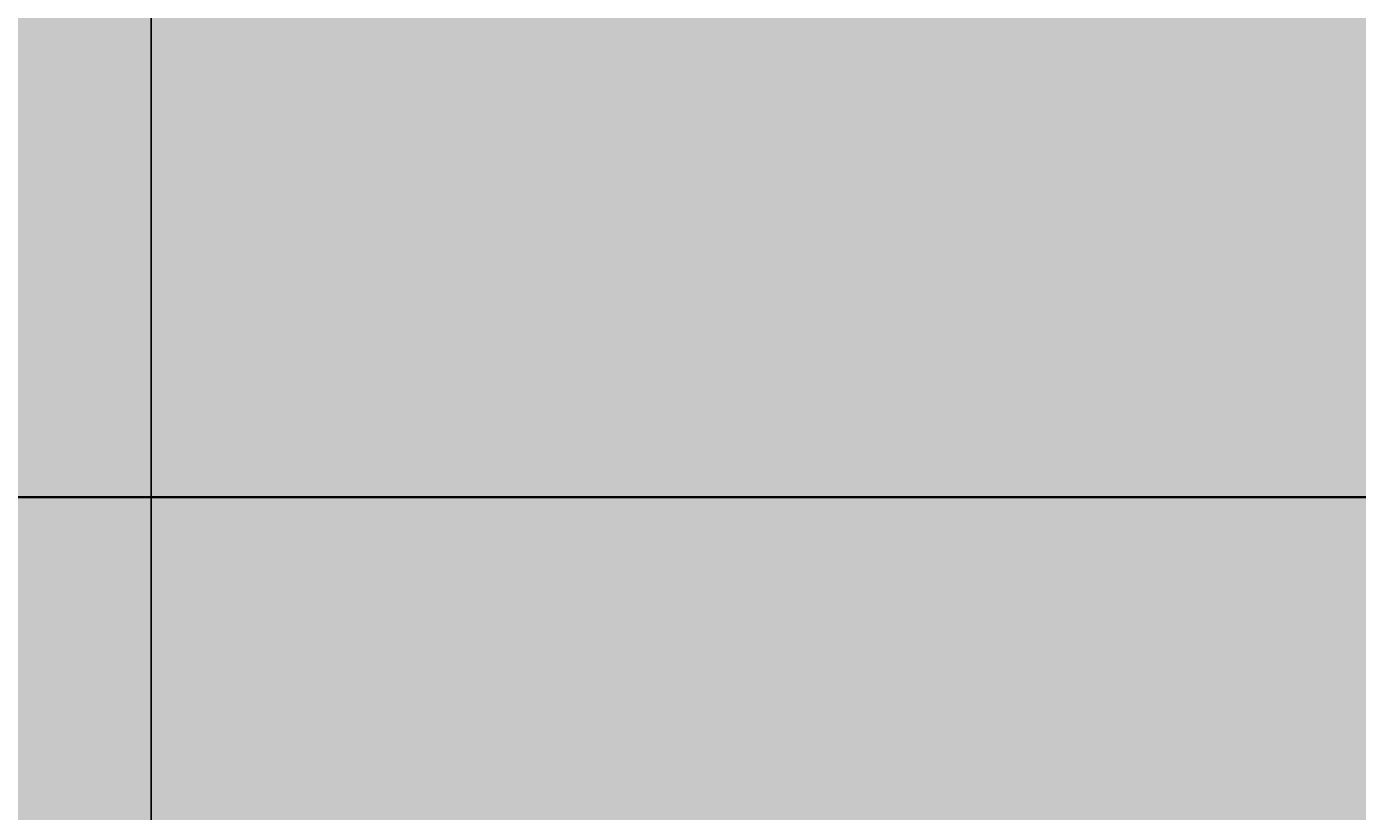
# Model space of a CAD drawing. Units: feet. Extents: x 2695 to 2912, y 795 to 1139.
# Tile 76 of 83: x 2840 to 2876, y 1042 to 1063. Entities that reach past the tile are written whole.
import ezdxf

# ---------------------------------------------------------------- set-up
doc = ezdxf.new("R2010")
doc.units = ezdxf.units.FT
for name, color, linetype, lineweight in [('A-ANNO-DIMS', 2, 'Continuous', 18), ('A-ELEV', 7, 'Continuous', 35), ('A-ELEV-PATT', 252, 'Continuous', 13)]:
    doc.layers.add(name, color=color, linetype=linetype, lineweight=lineweight)
doc.styles.get("Standard").update_dxf_attribs({"font": 'arial.ttf'})
doc.dimstyles.get("Standard").update_dxf_attribs({"dimtxt": 0.18, "dimasz": 0.18, "dimexe": 0.18, "dimexo": 0.0625, "dimgap": 0.09, "dimtad": 0, "dimtih": 1, "dimtoh": 1, "dimdec": 1, "dimzin": 0, "dimdsep": 46, "dimlunit": 3, "dimtxsty": 'Standard', "dimcen": 0.09, "dimadec": 0, "dimazin": 0, "dimtfac": 1, "dimtdec": 1, "dimtofl": 0, "dimtmove": 0, "dimatfit": 3, "dimfxl": 1, "dimtolj": 1, "dimtzin": 0, "dimarcsym": 0})

# ---------------------------------------------------------------- blocks, each defined once
blk = doc.blocks.new('*D10')
at = {"layer": 'A-ANNO-DIMS', "color": 0, "lineweight": -2, "transparency": 16777216}
for p, q in [((2778.034, 1020.886), (2778.034, 1138.886)), ((2778.214, 1138.706), (2810.411, 1138.706)), ((2843.395, 1138.706), (2811.198, 1138.706)), ((2843.575, 1020.886), (2843.575, 1138.886))]:
    blk.add_line(p, q, dxfattribs=at)
at = {"layer": 'A-ANNO-DIMS', "color": 0, "transparency": 16777216}
for points in [[(2778.214, 1138.736), (2778.214, 1138.676), (2778.034, 1138.706)], [(2843.395, 1138.736), (2843.395, 1138.676), (2843.575, 1138.706)]]:
    blk.add_solid(points, dxfattribs=at)
at = {"layer": 'Defpoints', "color": 0, "transparency": 16777216}
for p in [(2843.575, 1138.706), (2778.034, 1020.824), (2843.575, 1020.824)]:
    blk.add_point(p, dxfattribs=at)
at = {"layer": 'A-ANNO-DIMS', "color": 0, "transparency": 16777216, "insert": (2810.805, 1138.706), "char_height": 0.18, "attachment_point": 5}
blk.add_mtext('\\A1;65.54', dxfattribs=at)
blk = doc.blocks.new('*D11')
at = {"layer": 'A-ANNO-DIMS', "color": 0, "lineweight": -2, "transparency": 16777216}
for p, q in [((2843.575, 1020.886), (2843.575, 1138.886)), ((2843.755, 1138.706), (2869.128, 1138.706)), ((2895.289, 1138.706), (2869.916, 1138.706)), ((2895.469, 1107.898), (2895.469, 1138.886))]:
    blk.add_line(p, q, dxfattribs=at)
at = {"layer": 'A-ANNO-DIMS', "color": 0, "transparency": 16777216}
for points in [[(2843.755, 1138.736), (2843.755, 1138.676), (2843.575, 1138.706)], [(2895.289, 1138.736), (2895.289, 1138.676), (2895.469, 1138.706)]]:
    blk.add_solid(points, dxfattribs=at)
at = {"layer": 'Defpoints', "color": 0, "transparency": 16777216}
for p in [(2895.469, 1138.706), (2895.469, 1107.835), (2843.575, 1020.824)]:
    blk.add_point(p, dxfattribs=at)
at = {"layer": 'A-ANNO-DIMS', "color": 0, "transparency": 16777216, "insert": (2869.522, 1138.706), "char_height": 0.18, "attachment_point": 5}
blk.add_mtext('\\A1;51.89', dxfattribs=at)
blk = doc.blocks.new('*D18')
at = {"layer": 'A-ANNO-DIMS', "color": 0, "lineweight": -2, "transparency": 16777216}
for p, q in [((2890.699, 1050.311), (2911.424, 1050.311)), ((2911.244, 1050.131), (2911.244, 1035.749)), ((2911.244, 1021.004), (2911.244, 1035.385)), ((2843.637, 1020.824), (2911.424, 1020.824))]:
    blk.add_line(p, q, dxfattribs=at)
at = {"layer": 'A-ANNO-DIMS', "color": 0, "transparency": 16777216}
for points in [[(2911.214, 1050.131), (2911.274, 1050.131), (2911.244, 1050.311)], [(2911.214, 1021.004), (2911.274, 1021.004), (2911.244, 1020.824)]]:
    blk.add_solid(points, dxfattribs=at)
at = {"layer": 'Defpoints', "color": 0, "transparency": 16777216}
for p in [(2890.636, 1050.311), (2911.244, 1050.311), (2843.575, 1020.824)]:
    blk.add_point(p, dxfattribs=at)
at = {"layer": 'A-ANNO-DIMS', "color": 0, "transparency": 16777216, "insert": (2911.244, 1035.567), "char_height": 0.18, "attachment_point": 5}
blk.add_mtext('\\A1;29.487', dxfattribs=at)
blk = doc.blocks.new('*D50')
at = {"layer": 'A-ANNO-DIMS', "color": 0, "lineweight": -2, "transparency": 16777216}
for p, q in [((2810.041, 972.03), (2810.041, 1138.886)), ((2810.221, 1138.706), (2848.721, 1138.706)), ((2888.008, 1138.706), (2849.508, 1138.706)), ((2888.188, 972.03), (2888.188, 1138.886))]:
    blk.add_line(p, q, dxfattribs=at)
at = {"layer": 'A-ANNO-DIMS', "color": 0, "transparency": 16777216}
for points in [[(2810.221, 1138.736), (2810.221, 1138.676), (2810.041, 1138.706)], [(2888.008, 1138.736), (2888.008, 1138.676), (2888.188, 1138.706)]]:
    blk.add_solid(points, dxfattribs=at)
at = {"layer": 'Defpoints', "color": 0, "transparency": 16777216}
for p in [(2888.188, 1138.706), (2810.041, 971.967), (2888.188, 971.967)]:
    blk.add_point(p, dxfattribs=at)
at = {"layer": 'A-ANNO-DIMS', "color": 0, "transparency": 16777216, "insert": (2849.114, 1138.706), "char_height": 0.18, "attachment_point": 5}
blk.add_mtext('\\A1;78.15', dxfattribs=at)

msp = doc.modelspace()

# ---------------------------------------------------------------- hatches: boundary and pattern name
at = {"layer": 'A-ELEV-PATT'}
h = msp.add_hatch(color=256, dxfattribs=at)
h.set_gradient(color1=(255, 255, 255), tint=1)
h.paths.add_polyline_path([(2770.6361, 1122.9306), (2710.6361, 1122.9306), (2710.6361, 1118.4096), (2770.6361, 1118.4096)])
h.paths.add_polyline_path([(2890.6361, 1107.8588), (2770.6361, 1107.8588), (2770.6361, 1103.3378), (2890.6361, 1103.3378)])
h.paths.add_polyline_path([(2890.6361, 1062.9306), (2710.6361, 1062.9306), (2710.6361, 1056.9306), (2710.6361, 936.9306), (2710.6361, 924.3105), (2716.5358, 924.3105), (2890.6361, 924.3105), (2890.6361, 936.9306), (2715.8852, 936.9306), (2715.8852, 1050.3105), (2890.6361, 1050.3105)])
h.paths.add_polyline_path([(2716.5358, 924.3105), (2710.6361, 924.3105), (2710.6361, 810.9306), (2716.5358, 810.9306)])
h = msp.add_hatch(color=256, dxfattribs=at)
h.set_gradient(color1=(147, 149, 152), color2=(147, 149, 152), tint=1)
h.paths.add_polyline_path([(2770.6361, 1118.4096), (2710.6361, 1118.4096), (2710.6361, 1062.9306), (2770.6361, 1062.9306)])
h.paths.add_polyline_path([(2890.6361, 1103.3378), (2770.6361, 1103.3378), (2770.6361, 1062.9306), (2890.6361, 1062.9306)])
h.paths.add_polyline_path([(2730.7081, 1048.1052), (2755.1125, 1048.1052), (2755.1125, 936.9306), (2770.6361, 936.9306), (2770.6361, 1050.3105), (2715.8852, 1050.3105), (2715.8852, 936.9306), (2730.7081, 936.9306)])
h.paths.add_polyline_path([(2890.6361, 1050.3105), (2770.6361, 1050.3105), (2770.6361, 971.9673), (2778.0341, 971.9673), (2778.0341, 1020.8235), (2843.575, 1020.8235), (2843.575, 971.9673), (2890.6361, 971.9673)])
h.paths.add_polyline_path([(2888.1882, 970.7156), (2843.575, 970.7156), (2843.575, 964.8267), (2888.1882, 964.8267)])
h.paths.add_polyline_path([(2888.1882, 964.1328), (2843.575, 964.1328), (2843.575, 956.614), (2888.1882, 956.614)])
h.paths.add_polyline_path([(2888.1882, 955.9202), (2843.575, 955.9202), (2843.575, 949.2892), (2888.1882, 949.2892)])
h.paths.add_polyline_path([(2888.1882, 948.5954), (2843.575, 948.5954), (2843.575, 941.3507), (2888.1882, 941.3507)])
h.paths.add_polyline_path([(2888.1882, 940.6569), (2843.575, 940.6569), (2843.575, 936.9306), (2888.1882, 936.9306)])
h.paths.add_polyline_path([(2890.6361, 970.7156), (2888.9368, 970.7156), (2888.9368, 964.8267), (2890.6361, 964.8267)])
h.paths.add_polyline_path([(2890.6361, 964.1328), (2888.9368, 964.1328), (2888.9368, 956.614), (2890.6361, 956.614)])
h.paths.add_polyline_path([(2890.6361, 955.9202), (2888.9368, 955.9202), (2888.9368, 949.2892), (2890.6361, 949.2892)])
h.paths.add_polyline_path([(2890.6361, 940.6569), (2888.9368, 940.6569), (2888.9368, 936.9306), (2890.6361, 936.9306)])
h.paths.add_polyline_path([(2890.6361, 948.5954), (2888.9368, 948.5954), (2888.9368, 941.3507), (2890.6361, 941.3507)])
h.paths.add_polyline_path([(2772.5216, 970.7156), (2770.6361, 970.7156), (2770.6361, 964.8267), (2772.5216, 964.8267)])
h.paths.add_polyline_path([(2772.5216, 964.1328), (2770.6361, 964.1328), (2770.6361, 956.614), (2772.5216, 956.614)])
h.paths.add_polyline_path([(2772.5216, 955.9202), (2770.6361, 955.9202), (2770.6361, 949.2892), (2772.5216, 949.2892)])
h.paths.add_polyline_path([(2772.5216, 948.5954), (2770.6361, 948.5954), (2770.6361, 941.3507), (2772.5216, 941.3507)])
h.paths.add_polyline_path([(2772.5216, 940.6569), (2770.6361, 940.6569), (2770.6361, 936.9306), (2772.5216, 936.9306)])
h.paths.add_polyline_path([(2778.0341, 940.6569), (2773.2702, 940.6569), (2773.2702, 936.9306), (2778.0341, 936.9306)])
h.paths.add_polyline_path([(2778.0341, 970.7156), (2773.2702, 970.7156), (2773.2702, 964.8267), (2778.0341, 964.8267)])
h.paths.add_polyline_path([(2778.0341, 964.1328), (2773.2702, 964.1328), (2773.2702, 956.614), (2778.0341, 956.614)])
h.paths.add_polyline_path([(2778.0341, 955.9202), (2773.2702, 955.9202), (2773.2702, 949.2892), (2778.0341, 949.2892)])
h.paths.add_polyline_path([(2778.0341, 948.5954), (2773.2702, 948.5954), (2773.2702, 941.3507), (2778.0341, 941.3507)])
h.paths.add_polyline_path([(2810.0407, 940.6569), (2780.0341, 940.6569), (2780.0341, 936.9306), (2810.0407, 936.9306)])
h.paths.add_polyline_path([(2890.6361, 924.3105), (2770.6361, 924.3105), (2770.6361, 810.9306), (2773.5029, 810.9306), (2773.5029, 905.5143), (2805.9398, 905.5143), (2838.3767, 905.5143), (2838.3767, 810.9306), (2890.6361, 810.9306)])

# ---------------------------------------------------------------- linework, layer by layer
at = {"layer": 'A-ELEV'}
msp.add_line((2890.6361, 1050.3105), (2715.8852, 1050.3105), dxfattribs=at)
msp.add_lwpolyline([(2890.6361, 1050.3105), (2715.8852, 1050.3105)], dxfattribs=at)

# ---------------------------------------------------------------- dimensions: what is measured, and where the dimension line sits
at = {"layer": 'A-ANNO-DIMS'}
for base, p1, p2, picture, middle in [((2843.575, 1138.7056), (2778.0341, 1020.8235), (2843.575, 1020.8235), '*D10', (2810.8045, 1138.7056)), ((2888.1882, 1138.7056), (2810.0407, 971.9673), (2888.1882, 971.9673), '*D50', (2849.1144, 1138.7056)), ((2895.4694, 1138.7056), (2843.575, 1020.8235), (2895.4694, 1107.8352), '*D11', (2869.5222, 1138.7056))]:
    dim = msp.add_linear_dim(base=base, p1=p1, p2=p2, dimstyle='Standard', override={"dimdec": 2, "dimlfac": 1, "dimrnd": 0, "dimzin": 0, "dimdsep": 46, "dimlunit": 2}, dxfattribs=at)
    dim.commit()
    dim.dimension.update_dxf_attribs({"geometry": picture, "text_midpoint": middle})
dim = msp.add_linear_dim(base=(2911.2444, 1050.3105), p1=(2843.575, 1020.8235), p2=(2890.6361, 1050.3105), angle=90, dimstyle='Standard', override={"dimdec": 3, "dimlfac": 1, "dimrnd": 0, "dimzin": 0, "dimdsep": 46, "dimlunit": 2}, dxfattribs=at)
dim.commit()
dim.dimension.update_dxf_attribs({"geometry": '*D18', "text_midpoint": (2911.2444, 1035.567)})

doc.saveas('drawing.dxf')
